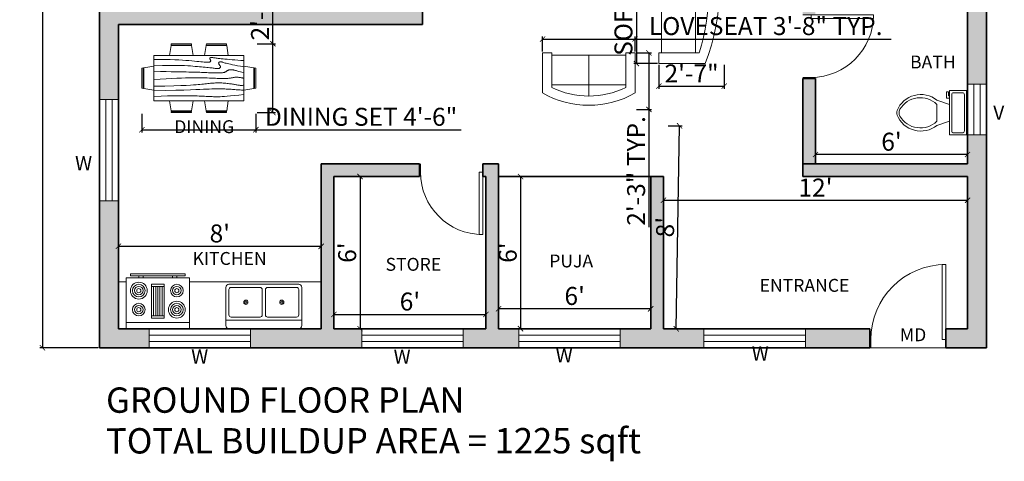
# Model space of a CAD drawing. Units: inches. Extents: x 3799 to 20199, y 1682 to 8087.
# Tile 4 of 30: x 8822 to 9289, y 1942 to 2151. Entities that reach past the tile are written whole.
import ezdxf

# ---------------------------------------------------------------- set-up
doc = ezdxf.new("R2010")
doc.units = ezdxf.units.IN
for name, color, linetype, lineweight in [('A-ANNO-DIMS', 2, 'Continuous', 18), ('A-ANNO-SYMB', 3, 'Continuous', 18), ('A-ANNO-TITL', 7, 'Continuous', 25), ('A-AREA-IDEN', 7, 'Continuous', 18), ('A-DOOR', 3, 'Continuous', 18), ('A-EQPM', 9, 'Continuous', 18), ('A-FLOR-CASE', 32, 'Continuous', 18), ('A-FLOR-FIXT', 9, 'Continuous', 18), ('A-FURN', 8, 'Continuous', 18), ('A-GLAZ', 152, 'Continuous', 18), ('A-WALL', 7, 'Continuous', 35), ('A-WALL-PATT', 252, 'Continuous', 13)]:
    doc.layers.add(name, color=color, linetype=linetype, lineweight=lineweight)
doc.styles.get("Standard").update_dxf_attribs({"font": 'arial.ttf'})
doc.dimstyles.new('ISO-25', dxfattribs={"dimtxt": 8.5, "dimasz": 2.5, "dimexe": 1.25, "dimexo": 0.625, "dimtad": 1, "dimdec": 0, "dimlunit": 3, "dimtxsty": 'Standard', "dimblk": 'ARCHTICK', "dimcen": 2.5, "dimadec": 0, "dimazin": 0, "dimtfac": 1, "dimtdec": 0, "dimtmove": 0, "dimatfit": 3, "dimfxl": 1, "dimarcsym": 0})

# ---------------------------------------------------------------- blocks, each defined once
blk = doc.blocks.new('*U23')
for p, q in [((-750, 0), (-750, 100)), ((0, 0), (0, 100))]:
    blk.add_line(p, q)
blk.add_lwpolyline([(0, 0), (0, -750), (-43.75, -750), (-43.75, 0)], close=True)
blk.add_arc((0, 0), 750, 180, 270)
blk = doc.blocks.new('*U7')
for p, q in [((0, 0), (0, -100)), ((750, 0), (750, -100))]:
    blk.add_line(p, q)
blk.add_lwpolyline([(0, 0), (0, 750), (43.75, 750), (43.75, 0)], close=True)
blk.add_arc((0, 0), 750, 0, 90)
blk = doc.blocks.new('*U22')
for p, q in [((0, 0), (0, -100)), ((-900, 0), (-900, -100))]:
    blk.add_line(p, q)
blk.add_lwpolyline([(0, 0), (0, 900), (-43.75, 900), (-43.75, 0)], close=True)
blk.add_arc((0, 0), 900, 90, 180)
blk = doc.blocks.new('Dining Set - 36 x 72 in.')
for p, q in [((-22.2343, 26.00059), (-23.4847, 17.99762)), ((-22.2304, 26), (-5.7608, 26)), ((-22, 27.5), (-22.1562, 26.50042)), ((-5.8416, 26.5), (-22.1534, 26.5)), ((-22, 27.5), (-6, 27.5)), ((-5.8437, 26.49966), (-6, 27.5)), ((-4.5152, 17.99762), (-5.7655, 25.99926)), ((5.7657, 26.00059), (4.5153, 17.99762)), ((5.7696, 26), (22.2392, 26)), ((6, 27.5), (5.8438, 26.50042)), ((22.1584, 26.5), (5.8466, 26.5)), ((6, 27.5), (22, 27.5)), ((22.1563, 26.49966), (22, 27.5)), ((23.4848, 17.99762), (22.2345, 25.99926)), ((36, 18), (-36, 18)), ((-36, 18), (-36, -18)), ((36, -18), (36, 18)), ((-45.5, 8), (-44.5004, 8.15617)), ((-45.5, 8), (-45.5, -8)), ((-44.5, -8.15843), (-44.5, 8.15338)), ((-44.0006, 8.23428), (-35.9976, 9.48474)), ((-44, 8.23041), (-44, -8.23915)), ((44.0006, 8.23428), (35.9976, 9.48474)), ((44, 8.23041), (44, -8.23915)), ((44.5, -8.15843), (44.5, 8.15338)), ((45.5, 8), (44.5005, 8.15617)), ((45.5, 8), (45.5, -8)), ((-44.4997, -8.15631), (-45.5, -8)), ((-35.9976, -9.48476), (-43.9993, -8.2345)), ((35.9976, -9.48476), (43.9993, -8.2345)), ((44.4997, -8.15631), (45.5, -8)), ((-36, -18), (36, -18)), ((-22.2343, -26.0006), (-23.4847, -17.99762)), ((-4.5152, -17.99762), (-5.7655, -25.99928)), ((5.7657, -26.0006), (4.5153, -17.99762)), ((23.4848, -17.99762), (22.2345, -25.99928)), ((-22.2304, -26), (-5.7608, -26)), ((-22, -27.5), (-22.1562, -26.50044)), ((-5.8416, -26.5), (-22.1534, -26.5)), ((-22, -27.5), (-6, -27.5)), ((-5.8437, -26.49967), (-6, -27.5)), ((5.7696, -26), (22.2392, -26)), ((6, -27.5), (5.8438, -26.50044)), ((22.1584, -26.5), (5.8466, -26.5)), ((6, -27.5), (22, -27.5)), ((22.1563, -26.49967), (22, -27.5))]:
    blk.add_line(p, q)
for points in [[(-36, 15), (-31.1772, 14.97754), (-26.8079, 14.91406), (-22.8538, 14.81543), (-19.276, 14.6875), (-16.0362, 14.53613), (-13.0957, 14.36718), (-10.4159, 14.18652), (-7.9583, 14), (-5.6904, 13.81315), (-3.6035, 13.63021), (-1.6954, 13.45508), (0.0365, 13.29166), (1.5945, 13.14388), (2.9811, 13.01562), (4.1988, 12.9108), (5.25, 12.83333), (6.1393, 12.78613), (6.8802, 12.76823), (7.4883, 12.77767), (7.9792, 12.8125), (8.3685, 12.87077), (8.6719, 12.95052), (8.9049, 13.0498), (9.0833, 13.16666), (9.2205, 13.29899), (9.3216, 13.44401), (9.3895, 13.59879), (9.4271, 13.76041), (9.4373, 13.92594), (9.4232, 14.09245), (9.3875, 14.257), (9.3333, 14.41666), (9.2638, 14.56917), (9.1836, 14.71484), (9.0975, 14.85465), (9.0104, 14.98958), (8.9272, 15.1206), (8.8529, 15.2487), (8.7922, 15.37483), (8.75, 15.5), (8.7305, 15.62467), (8.7344, 15.74739), (8.7617, 15.86621), (8.8125, 15.97916), (8.8867, 16.08431), (8.9844, 16.17968), (9.1055, 16.26334), (9.25, 16.33333), (9.4189, 16.38802), (9.6172, 16.42708), (9.8506, 16.45052), (10.125, 16.45833), (10.4463, 16.45052), (10.8203, 16.42708), (11.2529, 16.38802), (11.75, 16.33333), (12.3184, 16.26318), (12.9694, 16.17838), (13.7151, 16.07991), (14.5677, 15.96875), (15.5395, 15.84586), (16.6426, 15.71224), (17.8893, 15.56884), (19.2917, 15.41666), (20.859, 15.25667), (22.5879, 15.08984), (24.4721, 14.91715), (26.5052, 14.73958), (28.6809, 14.5581), (30.9929, 14.3737), (33.4347, 14.18733), (36, 14)], [(-36, 10), (-28.9766, 10.14274), (-23.1725, 10.20442), (-18.4241, 10.19775), (-14.5677, 10.13541), (-11.4399, 10.03011), (-8.877, 9.89453), (-6.7154, 9.74137), (-4.7917, 9.58333), (-2.9698, 9.43082), (-1.2246, 9.28515), (0.4415, 9.14534), (2.026, 9.01041), (3.5266, 8.87939), (4.9408, 8.7513), (6.266, 8.62516), (7.5, 8.5), (8.6411, 8.37549), (9.6914, 8.2539), (10.6538, 8.13818), (11.5312, 8.03125), (12.3267, 7.93603), (13.043, 7.85547), (13.6831, 7.79248), (14.25, 7.75), (14.7471, 7.7303), (15.1797, 7.73307), (15.5537, 7.75732), (15.875, 7.80208), (16.1494, 7.86637), (16.3828, 7.94922), (16.5811, 8.04964), (16.75, 8.16666), (16.8944, 8.29915), (17.0143, 8.44531), (17.1089, 8.60319), (17.1771, 8.77083), (17.218, 8.94629), (17.2305, 9.1276), (17.2137, 9.31282), (17.1667, 9.5), (17.0895, 9.6875), (16.987, 9.875), (16.8649, 10.0625), (16.7292, 10.25), (16.5856, 10.4375), (16.4401, 10.625), (16.2985, 10.8125), (16.1667, 11), (16.05, 11.18733), (15.9518, 11.3737), (15.8752, 11.5581), (15.8229, 11.73958), (15.798, 11.91715), (15.8034, 12.08984), (15.842, 12.25667), (15.9167, 12.41666), (16.0295, 12.56836), (16.1784, 12.70833), (16.3605, 12.83268), (16.5729, 12.9375), (16.8127, 13.01888), (17.0768, 13.07291), (17.3625, 13.0957), (17.6667, 13.08333), (17.9894, 13.03312), (18.3418, 12.94726), (18.7382, 12.82918), (19.1927, 12.68229), (19.7195, 12.51001), (20.3327, 12.31575), (21.0465, 12.10294), (21.875, 11.875), (22.8357, 11.63354), (23.959, 11.37304), (25.2786, 11.08618), (26.8282, 10.76562), (28.6414, 10.40405), (30.752, 9.99414), (33.1936, 9.52856), (36, 9)], [(-36, 5.5), (-30.7157, 5.3348), (-26.069, 5.20963), (-21.9946, 5.11767), (-18.4271, 5.05208), (-15.3009, 5.00602), (-12.5508, 4.97265), (-10.1112, 4.94515), (-7.9167, 4.91666), (-5.909, 4.88167), (-4.0586, 4.83984), (-2.3429, 4.79215), (-0.7396, 4.73958), (0.7739, 4.6831), (2.22, 4.6237), (3.6213, 4.56233), (5, 4.5), (6.373, 4.43782), (7.7344, 4.3776), (9.0723, 4.32129), (10.375, 4.27083), (11.6309, 4.22819), (12.8281, 4.19531), (13.9551, 4.17415), (15, 4.16666), (15.954, 4.17448), (16.819, 4.19791), (17.6001, 4.23698), (18.3021, 4.29166), (18.9299, 4.36198), (19.4883, 4.44791), (19.9823, 4.54948), (20.4167, 4.66666), (20.7969, 4.79899), (21.1302, 4.94401), (21.4245, 5.09879), (21.6875, 5.26041), (21.9271, 5.42594), (22.1511, 5.59245), (22.3672, 5.757), (22.5834, 5.91666), (22.8065, 6.06868), (23.0404, 6.21093), (23.2879, 6.34147), (23.5521, 6.45833), (23.8358, 6.55957), (24.142, 6.64323), (24.4735, 6.70735), (24.8334, 6.75), (25.2235, 6.76969), (25.642, 6.76692), (26.0858, 6.74267), (26.5521, 6.69791), (27.0379, 6.63362), (27.5404, 6.55078), (28.0565, 6.45036), (28.5834, 6.33333), (29.1242, 6.19987), (29.7071, 6.04687), (30.3661, 5.87044), (31.1354, 5.66666), (32.0493, 5.43164), (33.142, 5.16146), (34.4475, 4.85221), (36, 4.5)], [(-36, -1), (-30.7915, -0.6591), (-26.0195, -0.38216), (-21.6519, -0.16284), (-17.6563, 0.00521), (-14.0005, 0.12833), (-10.6523, 0.21289), (-7.5796, 0.26522), (-4.75, 0.29166), (-2.134, 0.29793), (0.2878, 0.28711), (2.5317, 0.26163), (4.6146, 0.22396), (6.5529, 0.17651), (8.3633, 0.12174), (10.0623, 0.06209), (11.6667, 0), (13.1899, -0.06201), (14.6341, -0.1211), (15.9982, -0.17432), (17.2813, -0.21875), (18.4823, -0.25147), (19.6003, -0.26953), (20.6343, -0.27002), (21.5834, -0.25), (22.4481, -0.20768), (23.2357, -0.14584), (23.9549, -0.06836), (24.6146, 0.02083), (25.2235, 0.11784), (25.7904, 0.21875), (26.3241, 0.31966), (26.8334, 0.41666), (27.3265, 0.50618), (27.8099, 0.58593), (28.2894, 0.65397), (28.7709, 0.70833), (29.2601, 0.74707), (29.763, 0.76823), (30.2855, 0.76985), (30.8334, 0.75), (31.4088, 0.70784), (31.9994, 0.64713), (32.589, 0.57275), (33.1615, 0.48958), (33.7008, 0.4025), (34.1908, 0.3164), (34.6153, 0.23616), (34.9584, 0.16666), (35.2099, 0.11165), (35.3848, 0.07031), (35.504, 0.04069), (35.5886, 0.02083), (35.6594, 0.00879), (35.7377, 0.0026), (35.8442, 0.00032), (36, 0)], [(-36, -6.5), (-27.1843, -6.31267), (-20.084, -6.1263), (-14.469, -5.9419), (-10.1094, -5.76042), (-6.7752, -5.58285), (-4.2363, -5.41016), (-2.2629, -5.24333), (-0.625, -5.08334), (0.8708, -4.93099), (2.2715, -4.78646), (3.5872, -4.64974), (4.8281, -4.52084), (6.0046, -4.39974), (7.127, -4.28646), (8.2053, -4.18099), (9.25, -4.08334), (10.2705, -3.99382), (11.2734, -3.91407), (12.2647, -3.84603), (13.25, -3.79167), (14.2354, -3.75293), (15.2266, -3.73177), (16.2295, -3.73015), (17.25, -3.75), (18.2912, -3.79248), (19.3451, -3.85547), (20.4009, -3.93604), (21.4479, -4.03125), (22.4754, -4.13819), (23.4727, -4.25391), (24.4289, -4.37549), (25.3334, -4.5), (26.1785, -4.62492), (26.9694, -4.74935), (27.7145, -4.87281), (28.4219, -4.99479), (29.1, -5.11483), (29.7572, -5.23242), (30.4016, -5.34709), (31.0417, -5.45834), (31.6837, -5.56437), (32.3262, -5.65821), (32.9658, -5.73153), (33.599, -5.77604), (34.2224, -5.78345), (34.8327, -5.74545), (35.4264, -5.65373), (36, -5.5)], [(-36, -10), (-26.4022, -9.81299), (-18.4675, -9.62891), (-11.9839, -9.45069), (-6.7396, -9.28125), (-2.5226, -9.12354), (0.8789, -8.98047), (3.6769, -8.85498), (6.0833, -8.75), (8.2767, -8.66765), (10.3021, -8.60677), (12.1712, -8.56543), (13.8958, -8.54167), (15.4876, -8.53353), (16.9583, -8.53907), (18.3197, -8.55632), (19.5834, -8.58334), (20.7616, -8.61841), (21.8685, -8.66081), (22.9188, -8.71004), (23.9271, -8.76563), (24.9081, -8.82707), (25.8763, -8.89388), (26.8465, -8.96558), (27.8334, -9.04167), (28.8474, -9.12118), (29.8828, -9.20117), (30.93, -9.27824), (31.9792, -9.34896), (33.0205, -9.40991), (34.0443, -9.45768), (35.0407, -9.48885), (36, -9.5)], [(-36, -14.5), (-30.0881, -14.33513), (-25.0332, -14.21224), (-20.7312, -14.12647), (-17.0781, -14.07292), (-13.97, -14.04671), (-11.3027, -14.04297), (-8.9724, -14.05681), (-6.875, -14.08334), (-4.9224, -14.11833), (-3.0905, -14.16016), (-1.3709, -14.20785), (0.2448, -14.26042), (1.7647, -14.3169), (3.1973, -14.3763), (4.5507, -14.43767), (5.8333, -14.5), (7.0554, -14.5621), (8.235, -14.62175), (9.3922, -14.67652), (10.5469, -14.72396), (11.7192, -14.76164), (12.929, -14.78711), (14.1965, -14.79794), (15.5417, -14.79167), (16.9933, -14.76424), (18.6152, -14.70508), (20.4804, -14.60197), (22.6615, -14.44271), (25.2312, -14.21509), (28.2624, -13.9069), (31.8277, -13.50594), (36, -13)]]:
    blk.add_lwpolyline(points)
blk = doc.blocks.new('Sofa - Roundback 7 ft.')
for p, q in [((-12.00002, -32.4421), (-12.00003, -6.5971)), ((11.99997, -32.4421), (11.99998, -6.5971)), ((-36.000027, -34), (-36.000027, -11.4696)), ((-35.999844, -13.3819), (35.9998, -13.3819)), ((35.99998, -34), (35.99998, -11.4696)), ((-36.000027, -32.4421), (35.99998, -32.4421))]:
    blk.add_line(p, q)
for points in [[(-36.000027, -34), (-42.000027, -34), (-42.000027, -8)], [(41.99998, -8), (41.99998, -34), (35.99998, -34)]]:
    blk.add_lwpolyline(points)
for centre, radius, start, end in [((0, -114.25), 114.25, 68.43141, 111.5686), ((-0.00001, -127.1968), 121.1968, 72.72033, 107.2797)]:
    blk.add_arc(centre, radius, start, end)
blk = doc.blocks.new('Sink-double - 36 in top')
for p, q in [((-18, -4), (18, -4)), ((-0.75, -18.5), (-0.75, -6.5)), ((0.75, -6.5), (0.75, -18.5))]:
    blk.add_line(p, q)
for points in [[(-16.5, 0), (16.5, 0)], [(-18, -19.5), (-18, -1.5)], [(18, -1.5), (18, -19.5)], [(-16.5, -18.5), (-16.5, -6.5)], [(-15.5, -5.5), (-1.75, -5.5)], [(1.75, -5.5), (15.5, -5.5)], [(16.5, -6.5), (16.5, -18.5)], [(16.5, -21), (-16.5, -21)], [(-1.75, -19.5), (-15.5, -19.5)], [(15.5, -19.5), (1.75, -19.5)]]:
    blk.add_lwpolyline(points)
for centre, radius in [((-8.5, -12.5), 1), ((-8.5, -12.5), 0.5), ((8.5, -12.5), 1), ((8.5, -12.5), 0.5)]:
    blk.add_circle(centre, radius)
for centre, radius, start, end in [((-16.5, -1.5), 1.5, 90, 180), ((16.5, -1.5), 1.5, 0, 90), ((-15.5, -6.5), 1, 90, 180), ((-1.75, -6.5), 1, 0, 90), ((1.75, -6.5), 1, 90, 180), ((15.5, -6.5), 1, 0, 90), ((-15.5, -18.5), 1, 180, 270), ((-1.75, -18.5), 1, 270, 0), ((1.75, -18.5), 1, 180, 270), ((15.5, -18.5), 1, 270, 0), ((-16.5, -19.5), 1.5, 180, 270), ((16.5, -19.5), 1.5, 270, 0)]:
    blk.add_arc(centre, radius, start, end)
blk = doc.blocks.new('Range-Oven - 30 in top')
for p, q in [((0, -3), (30, -3)), ((12, -6), (18, -6)), ((13, -20), (13, -6)), ((14, -6), (14, -20)), ((15, -20), (15, -6)), ((16, -6), (16, -20)), ((17, -20), (17, -6)), ((18, -20), (12, -20)), ((6, -24), (6, -25)), ((8, -25), (8, -24)), ((22, -25), (22, -24)), ((24, -24), (24, -25))]:
    blk.add_line(p, q)
for points in [[(0, -24), (0, 0), (30, 0), (30, -24)], [(12, -21), (12, -5), (18, -5), (18, -21)], [(2, -26), (2, -25), (28, -25), (28, -26)]]:
    blk.add_lwpolyline(points, close=True)
for centre, radius in [((6, -9), 4), ((6, -9), 3), ((6, -9), 2), ((6, -9), 1), ((24, -9), 3), ((24, -9), 2), ((24, -9), 1), ((6, -18), 3), ((6, -18), 2), ((6, -18), 1), ((24, -18), 4), ((24, -18), 3), ((24, -18), 2), ((24, -18), 1)]:
    blk.add_circle(centre, radius)
blk = doc.blocks.new('*U21')
for p, q in [((9.5, -6), (9.5, -2)), ((-10, -8.5), (-8, -8.5)), ((-10, -9.5), (-10, -8.5)), ((-8, -8.5), (-8, -8)), ((-7, -8), (-7, -9.5)), ((-4, -8), (-6, -14)), ((4, -8), (6, -14)), ((-7, -9.5), (-10, -9.5)), ((4, -14), (-4, -14))]:
    blk.add_line(p, q)
blk.add_lwpolyline([(10.5, -8), (10.5, 0), (-10.5, 0), (-10.5, -8)], close=True)
for points in [[(-9.5, -2), (-9.5, -6)], [(8.5, -1), (-8.5, -1)], [(-8.5, -7), (8.5, -7)]]:
    blk.add_lwpolyline(points)
for centre, radius, start, end in [((-8.62, -1.88), 0.884, 81.8699, 188.1301), ((8.62, -1.88), 0.884, 351.8699, 98.1301), ((-8.62, -6.12), 0.884, 171.8699, 278.1301), ((8.62, -6.12), 0.884, 261.8699, 8.1301), ((3.52, -21.58), 12.17, 141.4691, 247.9714), ((4.2, -21.82), 11.33, 136.3677, 238.9468), ((-3.52, -21.58), 12.17, 292.0284, 38.5307), ((-4.2, -21.82), 11.33, 301.053, 43.6321), ((0, -27.88), 4, 245.7318, 294.2682), ((0, -29), 4, 254.8605, 285.1395)]:
    blk.add_arc(centre, radius, start, end)
blk = doc.blocks.new('Sofa - Roundback Loveseat 5 ft.')
for p, q in [((0, -32.44198), (0, -5.99998)), ((-24, -33.99998), (-24, -11.46958)), ((24.00004, -33.99998), (24.00004, -11.46958)), ((-23.9998, -13.38178), (23.99986, -13.38178)), ((-24, -32.44198), (24.00004, -32.44198))]:
    blk.add_line(p, q)
for points in [[(-24, -33.99998), (-30, -33.99998), (-30, -7.99998)], [(30.00004, -7.99998), (30.00004, -33.99998), (24.00004, -33.99998)]]:
    blk.add_lwpolyline(points)
for centre, radius, start, end in [((0, -60.24998), 60.24998, 60.13715, 119.8628), ((0, -61.38438), 55.38444, 64.32083, 115.6792)]:
    blk.add_arc(centre, radius, start, end)
blk = doc.blocks.new('_ArchTick')
at = {"color": 0, "linetype": 'ByBlock', "const_width": 0.15}
blk.add_lwpolyline([(-0.5, -0.5), (0.5, 0.5)], dxfattribs=at)
blk = doc.blocks.new('*D32')
at = {"layer": 'A-ANNO-DIMS', "color": 0, "lineweight": -2, "transparency": 16777216}
for p, q in [((8859.58, 2415.42), (8831.97, 2415.42)), ((8833.22, 2415.42), (8833.22, 1995.42)), ((8859.58, 1995.42), (8831.97, 1995.42))]:
    blk.add_line(p, q, dxfattribs=at)
at = {"layer": 'Defpoints', "color": 0, "transparency": 16777216}
for p in [(8860.21, 2415.42), (8833.22, 1995.42), (8860.21, 1995.42)]:
    blk.add_point(p, dxfattribs=at)
at = {"layer": 'A-ANNO-DIMS', "color": 0, "lineweight": -2, "transparency": 16777216, "xscale": 2.5, "yscale": 2.5, "zscale": 2.5}
for p, rotation in [((8833.22, 2415.42), 90), ((8833.22, 1995.42), 270)]:
    blk.add_blockref('_ArchTick', p, dxfattribs=dict(at, rotation=rotation))
at = {"layer": 'A-ANNO-DIMS', "color": 0, "transparency": 16777216, "insert": (8828.25, 2205.42), "char_height": 8.5, "attachment_point": 5, "rotation": 90}
blk.add_mtext("35'", dxfattribs=at)
blk = doc.blocks.new('*D38')
at = {"layer": 'A-ANNO-DIMS', "color": 0, "lineweight": -2, "transparency": 16777216}
for p, q in [((9199.21, 2083.04), (9199.21, 2088.1)), ((9271.21, 2086.85), (9199.21, 2086.85)), ((9271.21, 2083.04), (9271.21, 2088.1))]:
    blk.add_line(p, q, dxfattribs=at)
at = {"layer": 'Defpoints', "color": 0, "transparency": 16777216}
for p in [(9199.21, 2086.85), (9199.21, 2082.42), (9271.21, 2082.42)]:
    blk.add_point(p, dxfattribs=at)
at = {"layer": 'A-ANNO-DIMS', "color": 0, "lineweight": -2, "transparency": 16777216, "xscale": 2.5, "yscale": 2.5, "zscale": 2.5, "rotation": 180}
blk.add_blockref('_ArchTick', (9199.21, 2086.85), dxfattribs=at)
at = {"layer": 'A-ANNO-DIMS', "color": 0, "lineweight": -2, "transparency": 16777216, "xscale": 2.5, "yscale": 2.5, "zscale": 2.5}
blk.add_blockref('_ArchTick', (9271.21, 2086.85), dxfattribs=at)
at = {"layer": 'A-ANNO-DIMS', "color": 0, "transparency": 16777216, "insert": (9235.21, 2091.81), "char_height": 8.5, "attachment_point": 5}
blk.add_mtext("6'", dxfattribs=at)
blk = doc.blocks.new('*D39')
at = {"layer": 'A-ANNO-DIMS', "color": 0, "lineweight": -2, "transparency": 16777216}
for p, q in [((9127.21, 2075.79), (9127.21, 2063.95)), ((9271.21, 2075.79), (9271.21, 2063.95)), ((9127.21, 2065.2), (9271.21, 2065.2))]:
    blk.add_line(p, q, dxfattribs=at)
at = {"layer": 'Defpoints', "color": 0, "transparency": 16777216}
for p in [(9127.21, 2076.42), (9271.21, 2076.42), (9271.21, 2065.2)]:
    blk.add_point(p, dxfattribs=at)
at = {"layer": 'A-ANNO-DIMS', "color": 0, "lineweight": -2, "transparency": 16777216, "xscale": 2.5, "yscale": 2.5, "zscale": 2.5, "rotation": 180}
blk.add_blockref('_ArchTick', (9127.21, 2065.2), dxfattribs=at)
at = {"layer": 'A-ANNO-DIMS', "color": 0, "lineweight": -2, "transparency": 16777216, "xscale": 2.5, "yscale": 2.5, "zscale": 2.5}
blk.add_blockref('_ArchTick', (9271.21, 2065.2), dxfattribs=at)
at = {"layer": 'A-ANNO-DIMS', "color": 0, "transparency": 16777216, "insert": (9199.21, 2070.1), "char_height": 8.5, "attachment_point": 5}
blk.add_mtext("12'", dxfattribs=at)
blk = doc.blocks.new('*D40')
at = {"layer": 'A-ANNO-DIMS', "color": 0, "lineweight": -2, "transparency": 16777216}
for p, q in [((9129.4, 2100.48), (9136.14, 2100.37)), ((9133.33, 2004.32), (9134.9, 2100.39)), ((9127.83, 2004.41), (9134.58, 2004.3))]:
    blk.add_line(p, q, dxfattribs=at)
at = {"layer": 'Defpoints', "color": 0, "transparency": 16777216}
for p in [(9128.78, 2100.49), (9134.9, 2100.39), (9127.21, 2004.42)]:
    blk.add_point(p, dxfattribs=at)
at = {"layer": 'A-ANNO-DIMS', "color": 0, "lineweight": -2, "transparency": 16777216, "xscale": 2.5, "yscale": 2.5, "zscale": 2.5}
for p, rotation in [((9134.9, 2100.39), 89.06477723431455), ((9133.33, 2004.32), 269.0647772343145)]:
    blk.add_blockref('_ArchTick', p, dxfattribs=dict(at, rotation=rotation))
at = {"layer": 'A-ANNO-DIMS', "color": 0, "transparency": 16777216, "insert": (9129.15, 2052.44), "char_height": 8.5, "attachment_point": 5, "rotation": 89.0648}
blk.add_mtext("8'", dxfattribs=at)
blk = doc.blocks.new('*D41')
at = {"layer": 'A-ANNO-DIMS', "color": 0, "lineweight": -2, "transparency": 16777216}
for p, q in [((9049.83, 2076.42), (9060.82, 2076.42)), ((9059.57, 2076.42), (9059.57, 2004.42)), ((9049.83, 2004.42), (9060.82, 2004.42))]:
    blk.add_line(p, q, dxfattribs=at)
at = {"layer": 'Defpoints', "color": 0, "transparency": 16777216}
for p in [(9049.21, 2076.42), (9049.21, 2004.42), (9059.57, 2004.42)]:
    blk.add_point(p, dxfattribs=at)
at = {"layer": 'A-ANNO-DIMS', "color": 0, "lineweight": -2, "transparency": 16777216, "xscale": 2.5, "yscale": 2.5, "zscale": 2.5}
for p, rotation in [((9059.57, 2076.42), 90), ((9059.57, 2004.42), 270)]:
    blk.add_blockref('_ArchTick', p, dxfattribs=dict(at, rotation=rotation))
at = {"layer": 'A-ANNO-DIMS', "color": 0, "transparency": 16777216, "insert": (9054.61, 2040.42), "char_height": 8.5, "attachment_point": 5, "rotation": 90}
blk.add_mtext("6'", dxfattribs=at)
blk = doc.blocks.new('*D42')
at = {"layer": 'A-ANNO-DIMS', "color": 0, "lineweight": -2, "transparency": 16777216}
for p, q in [((9049.21, 2005.04), (9049.21, 2015.08)), ((9121.21, 2013.83), (9049.21, 2013.83)), ((9121.21, 2005.04), (9121.21, 2015.08))]:
    blk.add_line(p, q, dxfattribs=at)
at = {"layer": 'Defpoints', "color": 0, "transparency": 16777216}
for p in [(9049.21, 2013.83), (9049.21, 2004.42), (9121.21, 2004.42)]:
    blk.add_point(p, dxfattribs=at)
at = {"layer": 'A-ANNO-DIMS', "color": 0, "lineweight": -2, "transparency": 16777216, "xscale": 2.5, "yscale": 2.5, "zscale": 2.5, "rotation": 180}
blk.add_blockref('_ArchTick', (9049.21, 2013.83), dxfattribs=at)
at = {"layer": 'A-ANNO-DIMS', "color": 0, "lineweight": -2, "transparency": 16777216, "xscale": 2.5, "yscale": 2.5, "zscale": 2.5}
blk.add_blockref('_ArchTick', (9121.21, 2013.83), dxfattribs=at)
at = {"layer": 'A-ANNO-DIMS', "color": 0, "transparency": 16777216, "insert": (9085.21, 2018.8), "char_height": 8.5, "attachment_point": 5}
blk.add_mtext("6'", dxfattribs=at)
blk = doc.blocks.new('*D43')
at = {"layer": 'A-ANNO-DIMS', "color": 0, "lineweight": -2, "transparency": 16777216}
for p, q in [((8971.21, 2005.04), (8971.21, 2012.45)), ((8971.21, 2011.2), (9043.21, 2011.2)), ((9043.21, 2005.04), (9043.21, 2012.45))]:
    blk.add_line(p, q, dxfattribs=at)
at = {"layer": 'Defpoints', "color": 0, "transparency": 16777216}
for p in [(9043.21, 2011.2), (8971.21, 2004.42), (9043.21, 2004.42)]:
    blk.add_point(p, dxfattribs=at)
at = {"layer": 'A-ANNO-DIMS', "color": 0, "lineweight": -2, "transparency": 16777216, "xscale": 2.5, "yscale": 2.5, "zscale": 2.5, "rotation": 180}
blk.add_blockref('_ArchTick', (8971.21, 2011.2), dxfattribs=at)
at = {"layer": 'A-ANNO-DIMS', "color": 0, "lineweight": -2, "transparency": 16777216, "xscale": 2.5, "yscale": 2.5, "zscale": 2.5}
blk.add_blockref('_ArchTick', (9043.21, 2011.2), dxfattribs=at)
at = {"layer": 'A-ANNO-DIMS', "color": 0, "transparency": 16777216, "insert": (9007.21, 2016.17), "char_height": 8.5, "attachment_point": 5}
blk.add_mtext("6'", dxfattribs=at)
blk = doc.blocks.new('*D44')
at = {"layer": 'A-ANNO-DIMS', "color": 0, "lineweight": -2, "transparency": 16777216}
for p, q in [((8971.83, 2076.42), (8984.83, 2076.42)), ((8983.58, 2076.42), (8983.58, 2004.42)), ((8971.83, 2004.42), (8984.83, 2004.42))]:
    blk.add_line(p, q, dxfattribs=at)
at = {"layer": 'Defpoints', "color": 0, "transparency": 16777216}
for p in [(8971.21, 2076.42), (8971.21, 2004.42), (8983.58, 2004.42)]:
    blk.add_point(p, dxfattribs=at)
at = {"layer": 'A-ANNO-DIMS', "color": 0, "lineweight": -2, "transparency": 16777216, "xscale": 2.5, "yscale": 2.5, "zscale": 2.5}
for p, rotation in [((8983.58, 2076.42), 90), ((8983.58, 2004.42), 270)]:
    blk.add_blockref('_ArchTick', p, dxfattribs=dict(at, rotation=rotation))
at = {"layer": 'A-ANNO-DIMS', "color": 0, "transparency": 16777216, "insert": (8978.61, 2040.42), "char_height": 8.5, "attachment_point": 5, "rotation": 90}
blk.add_mtext("6'", dxfattribs=at)
blk = doc.blocks.new('*D45')
at = {"layer": 'A-ANNO-DIMS', "color": 0, "lineweight": -2, "transparency": 16777216}
for p, q in [((8869.21, 2027.18), (8869.21, 2044.67)), ((8869.21, 2043.42), (8965.21, 2043.42)), ((8965.21, 2027.18), (8965.21, 2044.67))]:
    blk.add_line(p, q, dxfattribs=at)
at = {"layer": 'Defpoints', "color": 0, "transparency": 16777216}
for p in [(8965.21, 2043.42), (8869.21, 2026.55), (8965.21, 2026.55)]:
    blk.add_point(p, dxfattribs=at)
at = {"layer": 'A-ANNO-DIMS', "color": 0, "lineweight": -2, "transparency": 16777216, "xscale": 2.5, "yscale": 2.5, "zscale": 2.5, "rotation": 180}
blk.add_blockref('_ArchTick', (8869.21, 2043.42), dxfattribs=at)
at = {"layer": 'A-ANNO-DIMS', "color": 0, "lineweight": -2, "transparency": 16777216, "xscale": 2.5, "yscale": 2.5, "zscale": 2.5}
blk.add_blockref('_ArchTick', (8965.21, 2043.42), dxfattribs=at)
at = {"layer": 'A-ANNO-DIMS', "color": 0, "transparency": 16777216, "insert": (8917.21, 2048.39), "char_height": 8.5, "attachment_point": 5}
blk.add_mtext("8'", dxfattribs=at)
blk = doc.blocks.new('WIN-24IN-9IN-FRAME')
for p, q in [((0, 24), (9, 24)), ((3, 0), (3, 24)), ((6, 0), (6, 24)), ((0, 0), (9, 0))]:
    blk.add_line(p, q)
blk = doc.blocks.new('WIN-48IN-9IN-FRAME')
for p, q in [((0, 0), (0, 9)), ((48, 6), (0, 6)), ((48, 0), (48, 9)), ((48, 3), (0, 3))]:
    blk.add_line(p, q)
blk = doc.blocks.new('*D256')
at = {"layer": 'A-ANNO-DIMS', "color": 0, "lineweight": -2, "transparency": 16777216}
for p, q in [((9124.45, 2200.84), (9113.18, 2200.84)), ((9114.43, 2200.84), (9114.43, 2129.88)), ((9124.45, 2129.88), (9113.18, 2129.88))]:
    blk.add_line(p, q, dxfattribs=at)
at = {"layer": 'Defpoints', "color": 0, "transparency": 16777216}
for p in [(9125.08, 2200.84), (9114.43, 2129.88), (9125.08, 2129.88)]:
    blk.add_point(p, dxfattribs=at)
at = {"layer": 'A-ANNO-DIMS', "color": 0, "lineweight": -2, "transparency": 16777216, "xscale": 2.5, "yscale": 2.5, "zscale": 2.5}
for p, rotation in [((9114.43, 2200.84), 90), ((9114.43, 2129.88), 270)]:
    blk.add_blockref('_ArchTick', p, dxfattribs=dict(at, rotation=rotation))
at = {"layer": 'A-ANNO-DIMS', "color": 0, "transparency": 16777216, "insert": (9109.41, 2165.36), "char_height": 8.5, "attachment_point": 5, "rotation": 90}
blk.add_mtext('SOFA 5\'-11"', dxfattribs=at)
blk = doc.blocks.new('*D257')
at = {"layer": 'A-ANNO-DIMS', "color": 0, "lineweight": -2, "transparency": 16777216}
for p, q in [((9125.08, 2129.25), (9125.08, 2117.98)), ((9156.05, 2129.25), (9156.05, 2117.98)), ((9125.08, 2119.23), (9156.05, 2119.23))]:
    blk.add_line(p, q, dxfattribs=at)
at = {"layer": 'Defpoints', "color": 0, "transparency": 16777216}
for p in [(9125.08, 2129.88), (9156.05, 2129.88), (9156.05, 2119.23)]:
    blk.add_point(p, dxfattribs=at)
at = {"layer": 'A-ANNO-DIMS', "color": 0, "lineweight": -2, "transparency": 16777216, "xscale": 2.5, "yscale": 2.5, "zscale": 2.5, "rotation": 180}
blk.add_blockref('_ArchTick', (9125.08, 2119.23), dxfattribs=at)
at = {"layer": 'A-ANNO-DIMS', "color": 0, "lineweight": -2, "transparency": 16777216, "xscale": 2.5, "yscale": 2.5, "zscale": 2.5}
blk.add_blockref('_ArchTick', (9156.05, 2119.23), dxfattribs=at)
at = {"layer": 'A-ANNO-DIMS', "color": 0, "transparency": 16777216, "insert": (9140.57, 2124.12), "char_height": 8.5, "attachment_point": 5}
blk.add_mtext('2\'-7"', dxfattribs=at)
blk = doc.blocks.new('*D274')
at = {"layer": 'A-ANNO-DIMS', "color": 0, "lineweight": -2, "transparency": 16777216}
for p, q in [((9070, 2135.57), (9070, 2142.76)), ((9070, 2141.51), (9113.8, 2141.51)), ((9113.8, 2135.57), (9113.8, 2142.76)), ((9113.8, 2141.51), (9234.98, 2141.51))]:
    blk.add_line(p, q, dxfattribs=at)
at = {"layer": 'Defpoints', "color": 0, "transparency": 16777216}
for p in [(9113.8, 2141.51), (9070, 2134.94), (9113.8, 2134.94)]:
    blk.add_point(p, dxfattribs=at)
at = {"layer": 'A-ANNO-DIMS', "color": 0, "lineweight": -2, "transparency": 16777216, "xscale": 2.5, "yscale": 2.5, "zscale": 2.5, "rotation": 180}
blk.add_blockref('_ArchTick', (9070, 2141.51), dxfattribs=at)
at = {"layer": 'A-ANNO-DIMS', "color": 0, "lineweight": -2, "transparency": 16777216, "xscale": 2.5, "yscale": 2.5, "zscale": 2.5}
blk.add_blockref('_ArchTick', (9113.8, 2141.51), dxfattribs=at)
at = {"layer": 'A-ANNO-DIMS', "color": 0, "transparency": 16777216, "insert": (9175.64, 2146.54), "char_height": 8.5, "attachment_point": 5}
blk.add_mtext('LOVESEAT 3\'-8" TYP.', dxfattribs=at)
blk = doc.blocks.new('*D275')
at = {"layer": 'A-ANNO-DIMS', "color": 0, "lineweight": -2, "transparency": 16777216}
for p, q in [((9114.42, 2134.94), (9121.62, 2134.94)), ((9120.37, 2134.94), (9120.37, 2108.18)), ((9114.42, 2108.18), (9121.62, 2108.18)), ((9120.37, 2108.18), (9120.37, 2052.48))]:
    blk.add_line(p, q, dxfattribs=at)
at = {"layer": 'Defpoints', "color": 0, "transparency": 16777216}
for p in [(9113.8, 2134.94), (9113.8, 2108.18), (9120.37, 2108.18)]:
    blk.add_point(p, dxfattribs=at)
at = {"layer": 'A-ANNO-DIMS', "color": 0, "lineweight": -2, "transparency": 16777216, "xscale": 2.5, "yscale": 2.5, "zscale": 2.5}
for p, rotation in [((9120.37, 2134.94), 90), ((9120.37, 2108.18), 270)]:
    blk.add_blockref('_ArchTick', p, dxfattribs=dict(at, rotation=rotation))
at = {"layer": 'A-ANNO-DIMS', "color": 0, "transparency": 16777216, "insert": (9115.4, 2079.08), "char_height": 8.5, "attachment_point": 5, "rotation": 90}
blk.add_mtext('2\'-3" TYP.', dxfattribs=at)
blk = doc.blocks.new('*D288')
at = {"layer": 'A-ANNO-DIMS', "color": 0, "lineweight": -2, "transparency": 16777216}
for p, q in [((8880.32, 2106.05), (8880.32, 2097.33)), ((8934.26, 2106.05), (8934.26, 2097.33)), ((8880.32, 2098.58), (8934.26, 2098.58)), ((8934.26, 2098.58), (9031.44, 2098.58))]:
    blk.add_line(p, q, dxfattribs=at)
at = {"layer": 'Defpoints', "color": 0, "transparency": 16777216}
for p in [(8880.32, 2106.67), (8934.26, 2106.67), (8934.26, 2098.58)]:
    blk.add_point(p, dxfattribs=at)
at = {"layer": 'A-ANNO-DIMS', "color": 0, "lineweight": -2, "transparency": 16777216, "xscale": 2.5, "yscale": 2.5, "zscale": 2.5, "rotation": 180}
blk.add_blockref('_ArchTick', (8880.32, 2098.58), dxfattribs=at)
at = {"layer": 'A-ANNO-DIMS', "color": 0, "lineweight": -2, "transparency": 16777216, "xscale": 2.5, "yscale": 2.5, "zscale": 2.5}
blk.add_blockref('_ArchTick', (8934.26, 2098.58), dxfattribs=at)
at = {"layer": 'A-ANNO-DIMS', "color": 0, "transparency": 16777216, "insert": (8984.1, 2103.6), "char_height": 8.5, "attachment_point": 5}
blk.add_mtext('DINING SET 4\'-6"', dxfattribs=at)
blk = doc.blocks.new('*D289')
at = {"layer": 'A-ANNO-DIMS', "color": 0, "lineweight": -2, "transparency": 16777216}
for p, q in [((8942.35, 2139.27), (8942.35, 2185.57)), ((8934.89, 2139.27), (8943.6, 2139.27)), ((8942.35, 2106.67), (8942.35, 2139.27)), ((8934.89, 2106.67), (8943.6, 2106.67))]:
    blk.add_line(p, q, dxfattribs=at)
at = {"layer": 'Defpoints', "color": 0, "transparency": 16777216}
for p in [(8934.26, 2139.27), (8942.35, 2139.27), (8934.26, 2106.67)]:
    blk.add_point(p, dxfattribs=at)
at = {"layer": 'A-ANNO-DIMS', "color": 0, "lineweight": -2, "transparency": 16777216, "xscale": 2.5, "yscale": 2.5, "zscale": 2.5}
for p, rotation in [((8942.35, 2139.27), 90), ((8942.35, 2106.67), 270)]:
    blk.add_blockref('_ArchTick', p, dxfattribs=dict(at, rotation=rotation))
at = {"layer": 'A-ANNO-DIMS', "color": 0, "transparency": 16777216, "insert": (8937.34, 2163.67), "char_height": 8.5, "attachment_point": 5, "rotation": 90}
blk.add_mtext('2\'-8 1/2"', dxfattribs=at)

msp = doc.modelspace()

# ---------------------------------------------------------------- hatches: boundary and pattern name
at = {"layer": 'A-WALL-PATT'}
h = msp.add_hatch(color=256, dxfattribs=at)
h.dxf.hatch_style = 1
h.paths.add_polyline_path([(8869.21, 2406.42), (8941.21, 2406.42), (8941.21, 2400.8), (8947.21, 2400.8), (8947.21, 2406.42), (8990.79, 2406.42), (8990.79, 2415.42), (8860.21, 2415.42), (8860.21, 2344.29), (8869.21, 2344.29)])
h.paths.add_polyline_path([(8869.21, 2320.29), (8860.21, 2320.29), (8860.21, 2228.85), (8869.21, 2228.85), (8869.21, 2256.42), (9053.08, 2256.42), (9053.08, 2262.42), (8947.21, 2262.42), (8947.21, 2370.8), (8941.21, 2370.8), (8941.21, 2262.42), (8869.21, 2262.42)])
h.paths.add_polyline_path([(9151.38, 2415.42), (9038.79, 2415.42), (9038.79, 2406.42), (9091.21, 2406.42), (9091.21, 2262.42), (9089.08, 2262.42), (9089.08, 2256.42), (9097.21, 2256.42), (9099.67, 2256.42), (9099.67, 2262.42), (9097.21, 2262.42), (9097.21, 2406.42), (9151.38, 2406.42)])
h.paths.add_polyline_path([(9280.21, 2415.42), (9199.38, 2415.42), (9199.38, 2406.42), (9271.21, 2406.42), (9271.21, 2262.42), (9269.42, 2262.42), (9269.42, 2256.42), (9271.21, 2256.42), (9271.21, 2202.87), (9280.21, 2202.87)])
h.paths.add_polyline_path([(9280.21, 2178.87), (9271.21, 2178.87), (9271.21, 2160.42), (9175.21, 2160.42), (9175.21, 2256.42), (9239.42, 2256.42), (9239.42, 2262.42), (9135.67, 2262.42), (9135.67, 2256.42), (9169.21, 2256.42), (9169.21, 2154.42), (9193.21, 2154.42), (9193.21, 2152.89), (9199.21, 2152.89), (9199.21, 2154.42), (9271.21, 2154.42), (9271.21, 2120.19), (9280.21, 2120.19)])
h.paths.add_polyline_path([(9199.21, 2122.89), (9193.21, 2122.89), (9193.21, 2082.42), (9199.21, 2082.42)])
h.paths.add_polyline_path([(9146.43, 2004.42), (9127.21, 2004.42), (9127.21, 2076.42), (9121.21, 2076.42), (9121.21, 2004.42), (9106.79, 2004.42), (9106.79, 1995.42), (9146.43, 1995.42)])
h.paths.add_polyline_path([(9058.79, 2004.42), (9049.21, 2004.42), (9049.21, 2082.42), (9041.72, 2082.42), (9041.72, 2076.42), (9043.21, 2076.42), (9043.21, 2004.42), (9032.46, 2004.42), (9032.46, 1995.42), (9058.79, 1995.42)])
h.paths.add_polyline_path([(8984.46, 2004.42), (8971.21, 2004.42), (8971.21, 2076.42), (9011.72, 2076.42), (9011.72, 2082.42), (8965.21, 2082.42), (8965.21, 2004.42), (8931.73, 2004.42), (8931.73, 1995.42), (8984.46, 1995.42)])
h.paths.add_polyline_path([(8883.73, 2004.42), (8869.21, 2004.42), (8869.21, 2064.88), (8860.21, 2064.88), (8860.21, 1995.42), (8883.73, 1995.42)])
h.paths.add_polyline_path([(8869.21, 2148.42), (9013.21, 2148.42), (9013.21, 2154.42), (8869.21, 2154.42), (8869.21, 2180.85), (8860.21, 2180.85), (8860.21, 2112.88), (8869.21, 2112.88)])
h = msp.add_hatch(color=256, dxfattribs=at)
h.dxf.hatch_style = 1
h.paths.add_polyline_path([(9280.21, 2096.19), (9271.21, 2096.19), (9271.21, 2082.42), (9199.21, 2082.42), (9193.21, 2082.42), (9193.21, 2076.42), (9271.21, 2076.42), (9271.21, 2004.42), (9260.88, 2004.42), (9260.88, 1995.42), (9280.21, 1995.42)])
h.paths.add_polyline_path([(9224.88, 2004.42), (9194.43, 2004.42), (9194.43, 1995.42), (9224.88, 1995.42)], flags=17)

# ---------------------------------------------------------------- linework, layer by layer
at = {"layer": 'A-DOOR'}
msp.add_line((9260.88, 1995.42), (9224.88, 1995.42), dxfattribs=at)
at = {"layer": 'A-FLOR-CASE'}
for p, q in [((8872.86, 2026.55), (8869.21, 2026.55)), ((8965.21, 2026.55), (8902.86, 2026.55))]:
    msp.add_line(p, q, dxfattribs=at)
at = {"layer": 'A-WALL'}
for p, q in [((8860.21, 2415.42), (8860.21, 1995.42)), ((9280.21, 1995.42), (9280.21, 2415.42)), ((9013.21, 2148.42), (9013.21, 2154.42)), ((9271.21, 2082.42), (9271.21, 2154.42)), ((9013.21, 2148.42), (8869.21, 2148.42)), ((8869.21, 2148.42), (8869.21, 2004.42)), ((9193.21, 2076.42), (9193.21, 2122.89)), ((9193.21, 2122.89), (9199.21, 2122.89)), ((9199.21, 2082.42), (9199.21, 2122.89)), ((8965.21, 2082.42), (8965.21, 2004.42)), ((8965.21, 2082.42), (9011.72, 2082.42)), ((9011.72, 2076.42), (9011.72, 2082.42)), ((9041.72, 2076.42), (9041.72, 2082.42)), ((9041.72, 2082.42), (9049.21, 2082.42)), ((9049.21, 2082.42), (9049.21, 2004.42)), ((9193.21, 2082.42), (9271.21, 2082.42)), ((9271.21, 2082.42), (9199.21, 2082.42)), ((8971.21, 2076.42), (8971.21, 2004.42)), ((8971.21, 2076.42), (9011.72, 2076.42)), ((9041.72, 2076.42), (9043.21, 2076.42)), ((9043.21, 2076.42), (9043.21, 2004.42)), ((9049.21, 2076.42), (9127.21, 2076.42)), ((9121.21, 2076.42), (9121.21, 2004.42)), ((9127.21, 2004.42), (9127.21, 2076.42)), ((9271.21, 2076.42), (9193.21, 2076.42)), ((9193.21, 2076.42), (9271.21, 2076.42)), ((9193.21, 2076.42), (9271.21, 2076.42)), ((9271.21, 2004.42), (9271.21, 2076.42)), ((8869.21, 2004.42), (8965.21, 2004.42)), ((8971.21, 2004.42), (9043.21, 2004.42)), ((9049.21, 2004.42), (9121.21, 2004.42)), ((9127.21, 2004.42), (9224.88, 2004.42)), ((9224.88, 2004.42), (9224.88, 1995.42)), ((9260.88, 2004.42), (9260.88, 1995.42)), ((9260.88, 2004.42), (9271.21, 2004.42)), ((8860.21, 1995.42), (9224.88, 1995.42)), ((9260.88, 1995.42), (9280.21, 1995.42))]:
    msp.add_line(p, q, dxfattribs=at)

# ---------------------------------------------------------------- block references
at = {"layer": 'A-DOOR', "xscale": 0.0393700787401575, "yscale": 0.0393700787401575, "zscale": 0.0393700787401575, "rotation": 270}
msp.add_blockref('*U7', (9197.15, 2152.89), dxfattribs=at)
at = {"layer": 'A-DOOR', "xscale": 0.0393700787401575, "yscale": 0.0393700787401575, "zscale": 0.0393700787401575}
for name, p in [('*U23', (9041.72, 2078.48)), ('*U22', (9260.88, 1999.36))]:
    msp.add_blockref(name, p, dxfattribs=at)
at = {"layer": 'A-EQPM', "rotation": 180}
msp.add_blockref('Range-Oven - 30 in top', (8902.86, 2004.42), dxfattribs=at)
at = {"layer": 'A-FLOR-FIXT'}
for name, p, rotation in [('*U21', (9270.7, 2106.59), 270), ('Sink-double - 36 in top', (8938.05, 2004.42), 180)]:
    msp.add_blockref(name, p, dxfattribs=dict(at, rotation=rotation))
at = {"layer": 'A-FURN'}
for name, p, xscale, yscale, zscale, rotation in [('Sofa - Roundback 7 ft.', (9153.8, 2165.36), 0.8447815510693718, 0.8447815510693718, 0.8447815510693718, 270), ('Sofa - Roundback Loveseat 5 ft.', (9091.9, 2110.13), -0.729884385846111, 0.729884385846111, 0.729884385846111, 180)]:
    msp.add_blockref(name, p, dxfattribs=dict(at, xscale=xscale, yscale=yscale, zscale=zscale, rotation=rotation))
at = {"layer": 'A-FURN', "xscale": 0.5927666516427994, "yscale": 0.5927666516427994, "zscale": 0.5927666516427994}
msp.add_blockref('Dining Set - 36 x 72 in.', (8907.29, 2122.97), dxfattribs=at)
at = {"layer": 'A-GLAZ'}
for name, p in [('WIN-24IN-9IN-FRAME', (9271.21, 2096.19)), ('WIN-48IN-9IN-FRAME', (8883.73, 1995.42)), ('WIN-48IN-9IN-FRAME', (8984.46, 1995.42)), ('WIN-48IN-9IN-FRAME', (9058.79, 1995.42)), ('WIN-48IN-9IN-FRAME', (9146.43, 1995.42))]:
    msp.add_blockref(name, p, dxfattribs=at)
at = {"layer": 'A-GLAZ', "rotation": 90}
msp.add_blockref('WIN-48IN-9IN-FRAME', (8869.21, 2064.88), dxfattribs=at)

# ---------------------------------------------------------------- texts
at = {"layer": 'A-ANNO-SYMB'}
for s, height, p in [('V', 6.71, (9283.36, 2103.31)), ('W', 6.71, (8848.69, 2079.37)), ('MD', 6.1, (9239.19, 1998.49)), ('W', 6.71, (9076.22, 1988.48)), ('W', 6.71, (9169.05, 1989.34)), ('W', 6.71, (8903.66, 1987.88)), ('W', 6.71, (8999.5, 1987.82))]:
    msp.add_text(s, height=height, rotation=0.0167, dxfattribs=at).set_placement(p)
at = {"layer": 'A-ANNO-TITL'}
for s, p in [('GROUND FLOOR PLAN', (8863.35, 1964.61)), ('TOTAL BUILDUP AREA = 1225 sqft', (8863.35, 1945.33))]:
    msp.add_text(s, height=12, rotation=0.0167, dxfattribs=at).set_placement(p)
at = {"layer": 'A-AREA-IDEN'}
for s, p in [('BATH', (9244, 2127.59)), ('DINING', (8895.65, 2096.97)), ('KITCHEN', (8904.29, 2034.6)), ('STORE', (8995.69, 2031.82)), ('PUJA', (9073.17, 2033.42)), ('ENTRANCE', (9172.79, 2021.86))]:
    msp.add_text(s, height=6.1, rotation=0.0167, dxfattribs=at).set_placement(p)

# ---------------------------------------------------------------- dimensions: what is measured, and where the dimension line sits
at = {"layer": 'A-ANNO-DIMS'}
for base, p1, p2, override, picture, middle in [((8833.22, 1995.42), (8860.21, 2415.42), (8860.21, 1995.42), {"dimclrd": 0, "dimclre": 0, "dimclrt": 0}, '*D32', (8828.25, 2205.42)), ((8942.35, 2139.27), (8934.26, 2106.67), (8934.26, 2139.27), {"dimdec": 1, "dimlfac": 1, "dimrnd": 0, "dimzin": 1, "dimdsep": 46, "dimlunit": 4, "dimfrac": 2}, '*D289', (8937.34, 2163.67)), ((8983.58, 2004.42), (8971.21, 2076.42), (8971.21, 2004.42), {"dimclrd": 0, "dimclre": 0, "dimclrt": 0}, '*D44', (8978.61, 2040.42)), ((9059.57, 2004.42), (9049.21, 2076.42), (9049.21, 2004.42), {"dimclrd": 0, "dimclre": 0, "dimclrt": 0}, '*D41', (9054.61, 2040.42))]:
    dim = msp.add_linear_dim(base=base, p1=p1, p2=p2, angle=90, dimstyle='ISO-25', override=override, dxfattribs=at)
    dim.commit()
    dim.dimension.update_dxf_attribs({"geometry": picture, "text_midpoint": middle})
for base, p1, p2, text, picture, middle in [((9114.43, 2129.88), (9125.08, 2200.84), (9125.08, 2129.88), 'SOFA <>', '*D256', (9109.41, 2165.36)), ((9120.37, 2108.18), (9113.8, 2134.94), (9113.8, 2108.18), '<> TYP.', '*D275', (9115.4, 2079.08))]:
    dim = msp.add_linear_dim(base=base, p1=p1, p2=p2, angle=270, text=text, dimstyle='ISO-25', override={"dimdec": 1, "dimlfac": 1, "dimrnd": 0, "dimzin": 1, "dimdsep": 46, "dimlunit": 4, "dimfrac": 2}, dxfattribs=at)
    dim.commit()
    dim.dimension.update_dxf_attribs({"geometry": picture, "text_midpoint": middle})
for base, p1, p2, text, picture, middle in [((9113.8, 2141.51), (9070, 2134.94), (9113.8, 2134.94), 'LOVESEAT <> TYP.', '*D274', (9175.64, 2146.54)), ((8934.26, 2098.58), (8880.32, 2106.67), (8934.26, 2106.67), 'DINING SET <>', '*D288', (8984.1, 2103.6))]:
    dim = msp.add_linear_dim(base=base, p1=p1, p2=p2, text=text, dimstyle='ISO-25', override={"dimdec": 1, "dimlfac": 1, "dimrnd": 0, "dimzin": 1, "dimdsep": 46, "dimlunit": 4, "dimfrac": 2}, dxfattribs=at)
    dim.commit()
    dim.dimension.update_dxf_attribs({"geometry": picture, "text_midpoint": middle})
for base, p1, p2, override, picture, middle in [((9156.05, 2119.23), (9125.08, 2129.88), (9156.05, 2129.88), {"dimdec": 1, "dimlfac": 1, "dimrnd": 0, "dimzin": 1, "dimdsep": 46, "dimlunit": 4, "dimfrac": 2}, '*D257', (9140.57, 2124.12)), ((9199.21, 2086.85), (9271.21, 2082.42), (9199.21, 2082.42), {"dimclrd": 0, "dimclre": 0, "dimclrt": 0}, '*D38', (9235.21, 2091.81)), ((9271.21, 2065.2), (9127.21, 2076.42), (9271.21, 2076.42), {"dimclrd": 0, "dimclre": 0, "dimclrt": 0}, '*D39', (9199.21, 2070.1)), ((8965.21, 2043.42), (8869.21, 2026.55), (8965.21, 2026.55), {"dimclrd": 0, "dimclre": 0, "dimclrt": 0}, '*D45', (8917.21, 2048.39)), ((9049.21, 2013.83), (9121.21, 2004.42), (9049.21, 2004.42), {"dimclrd": 0, "dimclre": 0, "dimclrt": 0}, '*D42', (9085.21, 2018.8)), ((9043.21, 2011.2), (8971.21, 2004.42), (9043.21, 2004.42), {"dimclrd": 0, "dimclre": 0, "dimclrt": 0}, '*D43', (9007.21, 2016.17))]:
    dim = msp.add_linear_dim(base=base, p1=p1, p2=p2, dimstyle='ISO-25', override=override, dxfattribs=at)
    dim.commit()
    dim.dimension.update_dxf_attribs({"geometry": picture, "text_midpoint": middle})
dim = msp.add_aligned_dim(p1=(9127.21, 2004.42), p2=(9128.78, 2100.49), distance=-6.12, dimstyle='ISO-25', override={"dimclrd": 0, "dimclre": 0, "dimclrt": 0}, dxfattribs=at)
dim.commit()
dim.dimension.update_dxf_attribs({"geometry": '*D40', "text_midpoint": (9129.15, 2052.44)})

doc.saveas('drawing.dxf')
